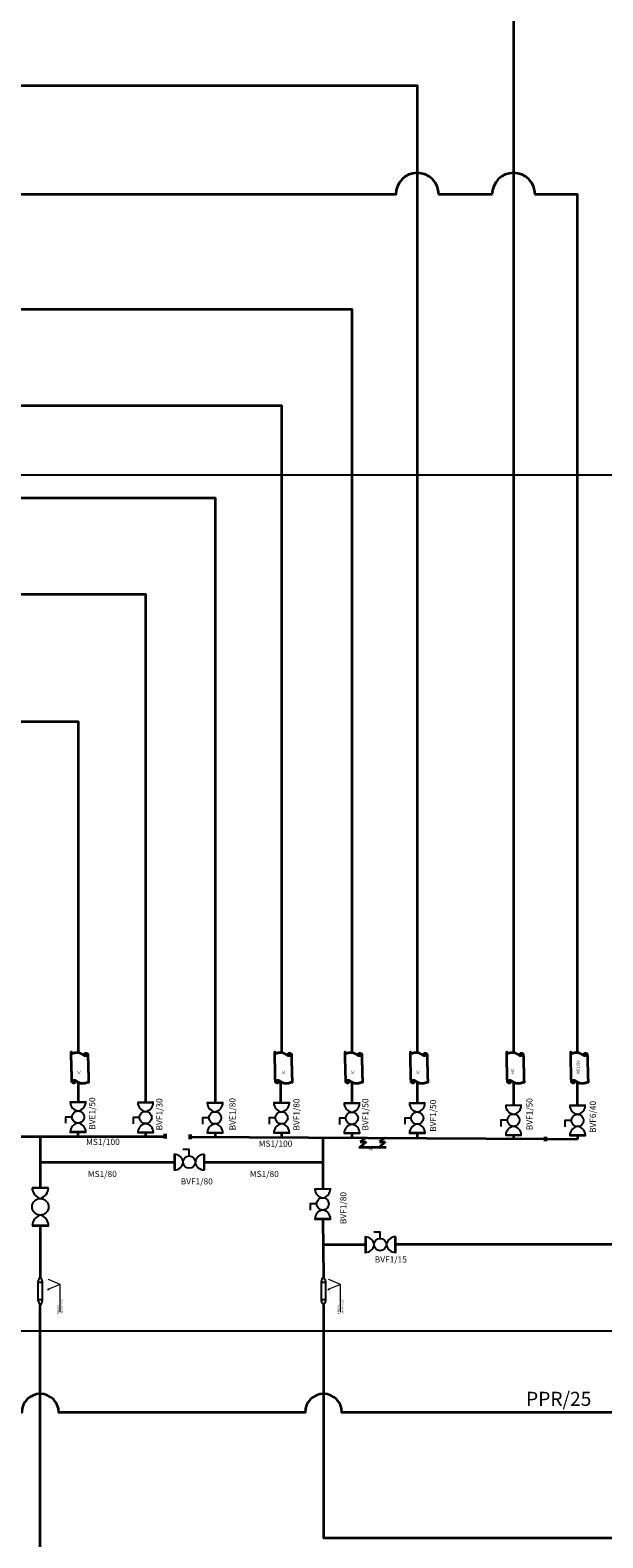
# Model space of a CAD drawing. Units: millimetres. Extents: x 353872 to 441597, y 126154 to 187356.
# Tile 4 of 28: x 372047 to 381210, y 143050 to 167178. Entities that reach past the tile are written whole.
import ezdxf

# ---------------------------------------------------------------- set-up
doc = ezdxf.new("R2010")
doc.units = ezdxf.units.MM
doc.linetypes.add('ACAD_ISO02W100', pattern=[15, 12, -3])
for name, color, linetype, lineweight in [('A-ANNO-DIMS', 2, 'Continuous', 18), ('P-ANNO-SYMB', 7, 'Continuous', 18), ('P-ANNO-TEXT', 7, 'Continuous', 25), ('P-BNDY', 4, 'ACAD_ISO02W100', 25), ('P-PIPE', 3, 'Continuous', 35), ('P-SYMB-PATT', 8, 'Continuous', 13), ('P-VALV', 2, 'Continuous', 25)]:
    doc.layers.add(name, color=color, linetype=linetype, lineweight=lineweight)
doc.styles.get("Standard").update_dxf_attribs({"font": 'arial.ttf'})
doc.dimstyles.get("Standard").update_dxf_attribs({"dimtxt": 0.18, "dimasz": 0.18, "dimexe": 0.18, "dimexo": 0.0625, "dimgap": 0.09, "dimtad": 0, "dimtih": 1, "dimtoh": 1, "dimdec": 4, "dimzin": 0, "dimdsep": 46, "dimtxsty": 'Standard', "dimcen": 0.09, "dimadec": 0, "dimazin": 0, "dimtfac": 1, "dimtdec": 4, "dimtofl": 0, "dimtmove": 0, "dimatfit": 3, "dimfxl": 1, "dimtolj": 1, "dimtzin": 0, "dimarcsym": 0})

# ---------------------------------------------------------------- blocks, each defined once
blk = doc.blocks.new('VALVE-A')
for points in [[(0, 9), (249, 9)], [(0, 6), (249, 6)], [(0, 3), (0, 0), (249, 0), (249, 4)], [(0, 3), (0, 3), (246, 3), (249, 3)]]:
    blk.add_lwpolyline(points)
for centre, radius, start, end in [((143, 1), 143, 97.3612, 180.5798), ((107, 2), 142, 359.2193, 82.8397)]:
    blk.add_arc(centre, radius, start, end)
blk = doc.blocks.new('VALVE-D-INDICATOR')
for points in [[(330, 249), (330, 0)], [(333, 249), (333, 0)], [(336, 249), (339, 249), (339, 0), (335, 0)], [(336, 249), (336, 246), (336, 3), (336, 0)]]:
    blk.add_lwpolyline(points)
blk.add_circle((98, 125), 98)
for centre, radius, start, end in [((338, 106), 143, 89.4202, 172.6388), ((337, 142), 142, 187.1603, 270.7807)]:
    blk.add_arc(centre, radius, start, end)
blk = doc.blocks.new('VALVE-F')
for points in [[(0, 9), (249, 9)], [(0, 6), (249, 6)], [(0, 3), (0, 0), (249, 0), (249, 4)], [(0, 3), (0, 3), (246, 3), (249, 3)], [(124, 143), (124, 143)]]:
    blk.add_lwpolyline(points)
for centre, radius, start, end in [((143, 1), 143, 97.3612, 180.5798), ((107, 2), 142, 359.2193, 82.8397)]:
    blk.add_arc(centre, radius, start, end)
blk = doc.blocks.new('PIPE-FITTING-A')
blk.add_arc((29, 49), 33.1, 215.9005, 359.7553)
for points, weights, knots in [([(0, 23), (0, 175), (0, 328), (0, 481), (36, 493), (109, 520), (173, 476), (205, 454), (216, 447), (228, 445), (240, 449), (252, 453), (261, 462), (265, 473)], [1, 1, 1, 1, 1, 1, 1, 1, 0.930126763637, 0.930126763637, 1, 0.930126763637, 0.930126763637, 1], [0, 0, 0, 0, 1, 1, 1, 33.012448, 65.874064, 65.874064, 65.874064, 66.797942, 66.797942, 66.797942, 67.721819, 67.721819, 67.721819, 67.721819]), ([(205, 454), (205, 469), (214, 481), (228, 486), (242, 490), (257, 485), (265, 473), (266, 473), (266, 472), (267, 471), (267, 321), (267, 172), (267, 23), (231, 10), (158, -17), (94, 27), (62, 49), (51, 56), (39, 58), (27, 54), (15, 50), (6, 42), (2, 30)], [1, 0.872926124327, 0.872926124327, 1, 0.872926124327, 0.872926124327, 1, 1, 1, 1, 1, 1, 1, 1, 1, 1, 1, 0.930126763637, 0.930126763637, 1, 0.930126763637, 0.930126763637, 1], [0, 0, 0, 0, 1.25537, 1.25537, 1.25537, 2.51074, 2.51074, 2.51074, 3.51074, 3.51074, 3.51074, 4.51074, 4.51074, 4.51074, 36.523189, 69.384804, 69.384804, 69.384804, 70.308682, 70.308682, 70.308682, 71.232559, 71.232559, 71.232559, 71.232559])]:
    blk.add_rational_spline(points, weights, degree=3, knots=knots)
blk = doc.blocks.new('VALVE-L')
for points in [[(0, 9), (264, 9)], [(0, 0), (264, 0), (264, 3)]]:
    blk.add_lwpolyline(points)
for centre, radius, start, end in [((204, -19), 205, 110.6617, 174.7476), ((86, 2), 178, 359.5088, 75.082)]:
    blk.add_arc(centre, radius, start, end)
blk = doc.blocks.new('PIPE-FITTING-B')
for p, q in [((95, 147), (0, 84)), ((0, 84), (95, 84)), ((95, 84), (0, 0))]:
    blk.add_line(p, q)
blk = doc.blocks.new('VALVE-P')
blk.add_lwpolyline([(264, 173), (0, 173)])
for centre, radius, start, end in [((199, 188), 200, 184.2463, 250.3444), ((64, 189), 201, 289.8639, 355.5453)]:
    blk.add_arc(centre, radius, start, end)
blk = doc.blocks.new('FLOW-ARROW')
blk.add_line((204, 86), (18, 7))
blk.add_lwpolyline([(15, 15), (21, 0), (0, 0)], close=True)
blk = doc.blocks.new('*D34')
at = {"layer": 'A-ANNO-DIMS', "color": 0, "lineweight": -2, "transparency": 16777216}
for p, q in [((399457, 167930), (356736, 167930)), ((356737, 167930), (356737, 163994)), ((356737, 160058), (356737, 163994)), ((399457, 160058), (356736, 160058))]:
    blk.add_line(p, q, dxfattribs=at)
at = {"layer": 'A-ANNO-DIMS', "color": 0, "transparency": 16777216}
for points in [[(356737, 167930), (356737, 167930), (356737, 167930)], [(356737, 160058), (356737, 160058), (356737, 160058)]]:
    blk.add_solid(points, dxfattribs=at)
at = {"layer": 'Defpoints', "color": 0, "transparency": 16777216}
for p in [(399457, 167930), (356737, 160058), (399457, 160058)]:
    blk.add_point(p, dxfattribs=at)
at = {"layer": 'A-ANNO-DIMS', "color": 0, "transparency": 16777216, "insert": (356737, 163994), "char_height": 0.18, "attachment_point": 5}
blk.add_mtext('\\A1;7872', dxfattribs=at)

msp = doc.modelspace()

# ---------------------------------------------------------------- hatches: boundary and pattern name
at = {"layer": 'P-SYMB-PATT'}
h = msp.add_hatch(color=256, dxfattribs=at)
h.dxf.hatch_style = 1
h.paths.add_polyline_path([(372322.83, 147020.96), (372343.58, 147020.96), (372337.34, 147035.79)])
h.paths.add_polyline_path([(372337.34, 147177.41), (372343.58, 147192.24), (372322.83, 147192.24)])
h = msp.add_hatch(color=256, dxfattribs=at)
h.dxf.hatch_style = 1
h.paths.add_polyline_path([(376809.72, 147020.96), (376830.47, 147020.96), (376824.23, 147035.79)])
h.paths.add_polyline_path([(376824.23, 147177.41), (376830.47, 147192.24), (376809.72, 147192.24)])

# ---------------------------------------------------------------- linework, layer by layer
at = {"layer": 'P-ANNO-SYMB'}
for points in [[(372526.57, 146661.43), (372526.57, 147106.6), (372340.46, 147184.83)], [(377013.46, 146661.43), (377013.46, 147106.6), (376827.35, 147184.83)]]:
    msp.add_lwpolyline(points, dxfattribs=at)
at = {"layer": 'P-BNDY'}
msp.add_line((360736.55, 146365.61), (391507.08, 146365.61), dxfattribs=at)
at = {"layer": 'P-PIPE'}
for p, q in [((369840.22, 149473.16), (374195.21, 149473.16)), ((372209.04, 149473.16), (372209.04, 148652.69)), ((372811.9, 149546.84), (372811.9, 149473.16)), ((373893.68, 149535.58), (373893.68, 149473.16)), ((374195.21, 149514.74), (374195.21, 149442.64)), ((374211.73, 149514.74), (374211.73, 149442.64)), ((374594.6, 149504.42), (374594.6, 149432.32)), ((374611.13, 149504.42), (374611.13, 149432.32)), ((374611.13, 149468.27), (380281, 149433.2)), ((375005.02, 149530.69), (375005.02, 149465.55)), ((376069.9, 149530.69), (376069.9, 149458.19)), ((376727.36, 149455.18), (376727.36, 148634.7)), ((377195.34, 149524.83), (377194.83, 149450.41)), ((378240.04, 149527.62), (378240.04, 149443.19)), ((379780.51, 149491.98), (379780.51, 149432.54)), ((380281, 149469.25), (380281, 149397.15)), ((380297.52, 149469.25), (380297.52, 149397.15)), ((380297.52, 149433.1), (380804.99, 149429.96)), ((380805, 149489.13), (380804.99, 149429.96)), ((377304.56, 149304.08), (377744.9, 149304.08)), ((372209.04, 149062.93), (374350.29, 149062.93)), ((374832.27, 149062.93), (376727.36, 149062.93)), ((376727.36, 148152.72), (376740.39, 147222.09)), ((372209.04, 148042.56), (372209.04, 147222.09)), ((376727.36, 147742.48), (377416.45, 147742.48))]:
    msp.add_line(p, q, dxfattribs=at)
for points in [[(366976.76, 171744.89), (381803.29, 171744.89), (381803.29, 150820.94), (381803.29, 147742.48), (377889.79, 147742.48)], [(366976.76, 170138.53), (379780.51, 170138.53), (379780.51, 150820.94)], [(366976.76, 166292.58), (378240.04, 166292.58), (378240.04, 150820.94)], [(368253.39, 162713.87), (377195.34, 162713.87), (377195.34, 150820.94)], [(366976.76, 161173.85), (376069.9, 161173.85), (376069.9, 150820.94)], [(366976.76, 159691.08), (375005.02, 159691.08), (375005.02, 150012.67)], [(366976.76, 158151.07), (373893.68, 158151.07), (373893.68, 150017.57)], [(366976.76, 156112.98), (372813.3, 156112.98), (372813.3, 150820.94)], [(372813.3, 150340.11), (372813.3, 150026.03)], [(376052.19, 150344.04), (376052.19, 150010.74)], [(377195.34, 150340.11), (377195.34, 150006.82)], [(378240.04, 150340.11), (378240.04, 150009.6)], [(379780.51, 150340.11), (379780.51, 149973.96)], [(380805, 149971.12), (380805, 150340.11)], [(376740.39, 146769.18), (376740.39, 143050.39), (379096.81, 143050.39), (382194.24, 143050.39)]]:
    msp.add_lwpolyline(points, dxfattribs=at)
for points in [[(380805, 150820.94), (380805, 164548.92), (380124.81, 164548.92, 1), (379436.2, 164548.92), (378584.35, 164548.92, 1), (377895.74, 164548.92), (366976.76, 164548.92)], [(379961.46, 141602.11), (378356.61, 141602.11, 1), (378244.32, 141602.11), (372209.04, 141602.11), (372209.04, 146769.18)], [(383301.45, 145058.64, 1), (382877.96, 145058.64), (377035.77, 145058.64, 1), (376445.02, 145058.64), (372504.41, 145058.64, 1), (371913.66, 145058.64), (366976.76, 145058.64)]]:
    msp.add_lwpolyline(points, format="xyb", dxfattribs=at)
at = {"layer": 'P-VALV'}
for points in [[(372714.94, 149785.03), (372612.3, 149785.03), (372612.3, 149684.25)], [(373795.33, 149776.58), (373692.68, 149776.58), (373692.68, 149675.8)], [(374906.66, 149771.68), (374804.01, 149771.68), (374804.01, 149670.9)], [(375971.54, 149771.68), (375868.9, 149771.68), (375868.9, 149670.9)], [(377096.99, 149765.82), (376994.34, 149765.82), (376994.34, 149665.04)], [(378141.69, 149768.61), (378039.04, 149768.61), (378039.04, 149667.83)], [(379682.15, 149732.97), (379579.51, 149732.97), (379579.51, 149632.19)], [(380706.64, 149730.13), (380604, 149730.13), (380604, 149629.35)], [(374591.28, 149161.28), (374591.28, 149263.93), (374490.5, 149263.93)], [(372340.02, 148643.62), (372078.02, 148643.62)], [(376629, 148393.71), (376526.36, 148393.71), (376526.36, 148292.93)], [(377648.8, 147840.85), (377648.8, 147943.49), (377548.02, 147943.49)], [(372171.65, 147147.09), (372171.65, 146851.71)], [(372246.42, 146851.71), (372246.42, 147147.09)], [(376703.01, 147147.09), (376703.01, 146851.71)], [(376777.78, 146851.71), (376777.78, 147147.09)]]:
    msp.add_lwpolyline(points, dxfattribs=at)
for centre, radius in [((372812.97, 149785.03), 98.03), ((373893.35, 149776.58), 98.03), ((375004.68, 149771.68), 98.03), ((376069.57, 149771.68), 98.03), ((377195.01, 149765.82), 98.03), ((378239.71, 149768.61), 98.03), ((379780.18, 149732.97), 98.03), ((380804.67, 149730.13), 98.03), ((372209.04, 148347.63), 131.9), ((376727.03, 148393.71), 98.03)]:
    msp.add_circle(centre, radius, dxfattribs=at)
for centre, radius, start, end in [((372308.92, 147125.48), 138.95, 135.955431, 171.055892), ((372050.94, 147096.46), 201.93, 14.518576, 38.470101), ((376840.27, 147125.48), 138.95, 135.955431, 171.055892), ((376582.29, 147096.46), 201.93, 14.518576, 38.470101), ((372209.04, 147247.51), 107.16, 249.581721, 290.418279), ((376740.39, 147247.51), 107.16, 249.581721, 290.418279), ((372209.04, 146773.25), 86.91, 64.522552, 115.477448), ((372414.36, 146911.92), 250.06, 193.932909, 214.806916), ((372210.79, 146757.55), 32.64, 71.051891, 113.980683), ((372017.65, 146905.61), 235.03, 324.517399, 346.742776), ((376740.39, 146773.25), 86.91, 64.522552, 115.477448), ((376945.71, 146911.92), 250.06, 193.932909, 214.806916), ((376742.14, 146757.55), 32.64, 71.051891, 113.980683), ((376549.01, 146905.61), 235.03, 324.517399, 346.742776)]:
    msp.add_arc(centre, radius, start, end, dxfattribs=at)

# ---------------------------------------------------------------- block references
at = {"layer": 'P-ANNO-SYMB'}
for p in [(372322.83, 147020.96), (376809.72, 147020.96)]:
    msp.add_blockref('FLOW-ARROW', p, dxfattribs=at)
at = {"layer": 'P-PIPE'}
for p, rotation in [((372715.45, 150314.09), 1.588978313901199), ((375972.05, 150314.09), 1.588978313767688), ((377097.49, 150314.09), 1.588978313901199), ((378142.19, 150314.09), 1.588978313796592), ((379682.65, 150314.09), 1.588978313778469), ((380707.15, 150314.09), 1.588978313842472)]:
    msp.add_blockref('PIPE-FITTING-A', p, dxfattribs=dict(at, rotation=rotation))
for p in [(377325.31, 149304.08), (377634.09, 149304.08)]:
    msp.add_blockref('PIPE-FITTING-B', p, dxfattribs=at)
at = {"layer": 'P-VALV'}
for name, p, rotation in [('VALVE-A', (372937.13, 150028.85), 181.3019170020567), ('VALVE-A', (374017.51, 150020.39), 181.3019170020399), ('VALVE-A', (375128.84, 150015.5), 181.3019170020267), ('VALVE-A', (376193.73, 150015.5), 181.3019170020304), ('VALVE-F', (377318.93, 150009.53), 181.2525321958925), ('VALVE-A', (378363.87, 150012.43), 181.3019170020567), ('VALVE-A', (379904.33, 149976.79), 181.3019170020304), ('VALVE-F', (380928.58, 149973.83), 181.252532195875), ('VALVE-A', (374350.29, 149187.3), 269.9999999998997), ('VALVE-A', (376851.19, 148637.53), 181.3019170020567), ('VALVE-A', (377407.8, 147866.86), 269.999999999835)]:
    msp.add_blockref(name, p, dxfattribs=dict(at, rotation=rotation))
for name, p in [('VALVE-A', (372688.93, 149544.04)), ('VALVE-A', (373769.31, 149535.58)), ('VALVE-A', (374880.64, 149530.69)), ('VALVE-A', (375945.53, 149530.69)), ('VALVE-F', (377070.97, 149524.83)), ('VALVE-A', (378115.67, 149527.62)), ('VALVE-F', (379656.13, 149491.98)), ('VALVE-F', (380680.63, 149489.13)), ('VALVE-D-INDICATOR', (374493.26, 148938.55)), ('VALVE-P', (372077.14, 148479.52)), ('VALVE-L', (372077.14, 148042.56)), ('VALVE-A', (376602.99, 148152.72)), ('VALVE-D-INDICATOR', (377550.77, 147618.11))]:
    msp.add_blockref(name, p, dxfattribs=at)

# ---------------------------------------------------------------- texts
at = {"layer": 'P-ANNO-TEXT'}
for s, height, p in [('IVF1/50', 46.014, (380838.86, 150471.74)), ('IC', 46.014, (372850.65, 150471.74)), ('IC', 46.014, (376124.92, 150471.74)), ('IC', 46.014, (377230.72, 150471.74)), ('IC', 46.014, (378271.36, 150471.74)), ('HC', 46.014, (379789.39, 150471.74)), ('BVE1/50', 98.09, (373088.15, 149580.58)), ('BVF1/30', 98.09, (374163.65, 149570.43)), ('BVE1/80', 98.09, (375332.66, 149570.43)), ('BVF1/80', 98.09, (376355.98, 149568.27)), ('BVF1/50', 98.09, (377458.9, 149568.27)), ('BVF1/50', 98.09, (380084.66, 149573.85)), ('BVF1/50', 98.09, (378542.42, 149548.64)), ('BVF6/40', 98.09, (381098.82, 149528.95)), ('BVF1/80', 98.09, (377105.42, 148070.97)), ('REDUCER', 22.559, (372502.31, 146629.8)), ('100 X 50(MS1)(2)', 22.5593, (372568.65, 146629.8)), ('REDUCER', 22.559, (376989.2, 146629.8)), ('100 X 50(MS1)(2)', 22.5593, (377055.54, 146629.8))]:
    msp.add_text(s, height=height, rotation=90, dxfattribs=at).set_placement(p)
for s, height, p in [('MS1/100', 98.09, (372941.91, 149337.78)), ('MS1/100', 98.09, (375703.63, 149309.89)), ('1HC', 27.7, (377458.49, 149251.49)), ('MS1/80', 98.09, (372969.82, 148824.65)), ('MS1/80', 98.09, (375561.97, 148824.65)), ('BVF1/80', 98.09, (374455.45, 148705.98)), ('BVF1/15', 98.09, (377560.02, 147456.93)), ('PPR/25', 225.086, (379981.12, 145162.21))]:
    msp.add_text(s, height=height, dxfattribs=at).set_placement(p)

# ---------------------------------------------------------------- dimensions: what is measured, and where the dimension line sits
at = {"layer": 'A-ANNO-DIMS'}
dim = msp.add_linear_dim(base=(356736.55, 160058.19), p1=(399457.15, 167929.97), p2=(399457.15, 160058.19), angle=90, dimstyle='Standard', override={"dimdec": 0, "dimlfac": 1, "dimrnd": 0, "dimzin": 0, "dimdsep": 46, "dimlunit": 2}, dxfattribs=at)
dim.commit()
dim.dimension.update_dxf_attribs({"geometry": '*D34', "text_midpoint": (356736.55, 163994.08)})

doc.saveas('drawing.dxf')
